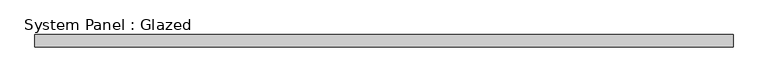
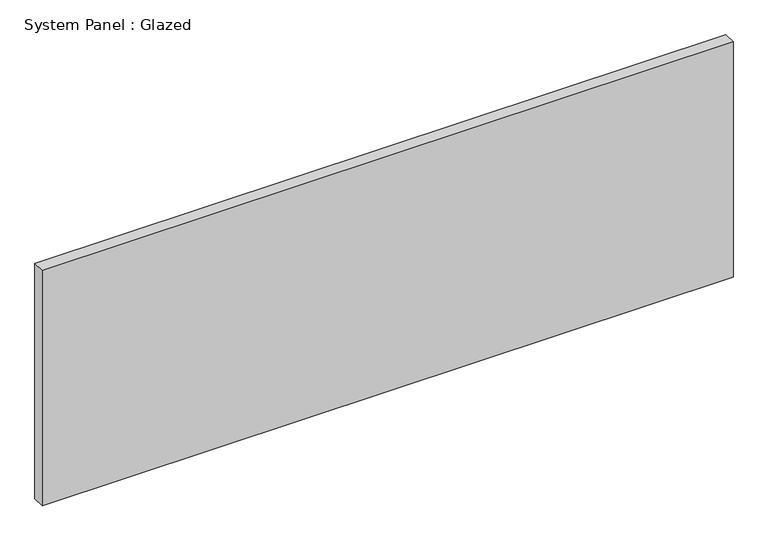
"""IFC4 building model written with IfcOpenShell, lengths in millimetres: plate geometry, System Panel : Glazed."""

from ifc_helpers import new_model, si_unit, origin, origin_with_axes, place, context, project, spatial, polyline, outline, extrude, source, transform, mapped, element, save


def system_panel_glazed_28169b10(model_context):
    return source(origin(), model_context, "Body", "SweptSolid", [
        extrude(outline(polyline([(714.3750001, 19.05), (-714.3750001, 19.05), (-714.3750001, 44.45), (714.3750001, 44.45), (714.3750001, 19.05)])), origin_with_axes(), (0.0, 0.0, 1.0), 514.35),
    ])


if __name__ == "__main__":
    model = new_model("IFC4")
    model_context = context("Model", 3, world=origin())
    ifc_project = project(units=[si_unit("LENGTHUNIT", "METRE", prefix="MILLI")], contexts=[model_context])
    site = spatial("IfcSite", under=ifc_project)
    building = spatial("IfcBuilding", under=site)
    placement = place(None, origin())
    system_panel_glazed_shape = system_panel_glazed_28169b10(model_context)
    element("IfcPlate", 1, ObjectType="System Panel : Glazed", at=placement, inside=building, context=model_context, shape_type="MappedRepresentation", body=[
        mapped(system_panel_glazed_shape, transform((0.0, 0.0, 0.0), x_axis=(1.0, 0.0, 0.0), y_axis=(0.0, 1.0, 0.0), z_axis=(0.0, 0.0, 1.0))),
    ])
    save(model, "model.ifc")

# Revit data of these elements
# Type "System Panel : Glazed"
#   Construction Type Id = "GSP4R"
#   Analytic Construction = "1/8 in Pilkington single glazing"
#   Visual Light Transmittance = 0.9
#   Solar Heat Gain Coefficient = 0.86
#   Heat Transfer Coefficient (U) = 1.18115 BTU/(h·ft²·°F)
#   Define Thermal Properties by = 1
# Element 1 (IfcPlate, "System Panel : Glazed")
#   Materials on its faces: "Glass"
# Materials
#   "Glass": class "Glass", colour RGB 0 128 192, transparency 0.75, Description = "Soda Lime Glass", Cost = 0
